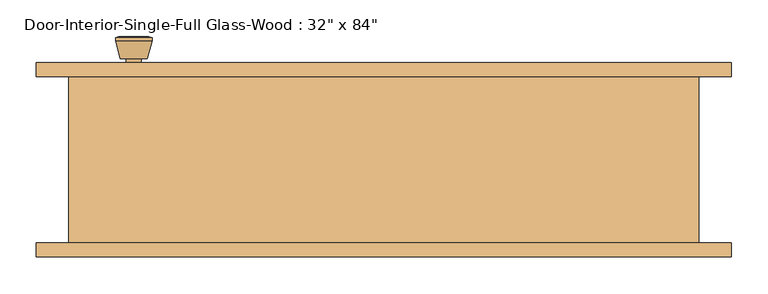
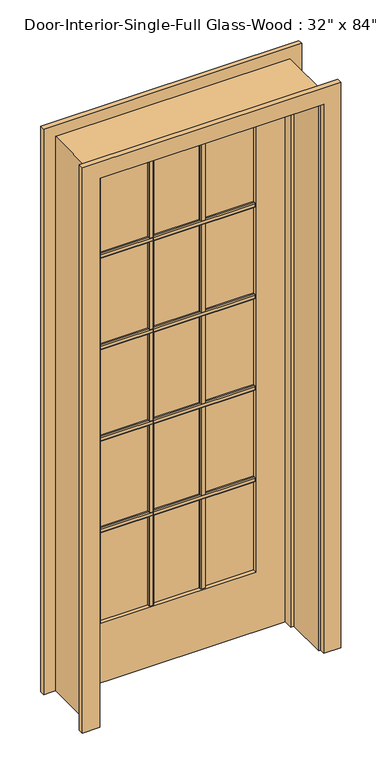
"""IFC4 building model written with IfcOpenShell, lengths in millimetres: door geometry."""

from ifc_helpers import new_model, si_unit, point, frame, frame_2d, origin, place, context, project, spatial, polyline, circle_curve, trimmed, segment, composite_curve, outline, extrude, faceted_brep, source, transform, mapped, element, save
from ifc_brep_helpers import plane_surface, cylinder_surface, revolved_surface, advanced_brep


def door_c0815308(model_context):
    return source(origin(), model_context, "Body", "SolidModel", [
        extrude(outline(polyline([(97.155, 1667.51), (103.505, 1667.51), (106.68, 1664.335), (106.68, 1651.635), (103.505, 1648.46), (97.155, 1648.46), (97.155, 1667.51)])), frame((-285.75, 0.0, 0.0), z_axis=(1.0, 0.0, 0.0), x_axis=(0.0, 1.0, 0.0)), (0.0, 0.0, 1.0), 571.5),
        extrude(outline(polyline([(97.155, 1310.9575), (103.505, 1310.9575), (106.68, 1307.7825), (106.68, 1295.0825), (103.505, 1291.9075), (97.155, 1291.9075), (97.155, 1310.9575)])), frame((-285.75, 0.0, 0.0), z_axis=(1.0, 0.0, 0.0), x_axis=(0.0, 1.0, 0.0)), (0.0, 0.0, 1.0), 571.5),
        extrude(outline(polyline([(97.155, 954.405), (103.505, 954.405), (106.68, 951.23), (106.68, 938.53), (103.505, 935.355), (97.155, 935.355), (97.155, 954.405)])), frame((-285.75, 0.0, 0.0), z_axis=(1.0, 0.0, 0.0), x_axis=(0.0, 1.0, 0.0)), (0.0, 0.0, 1.0), 571.5),
        extrude(outline(polyline([(97.155, 597.8525), (103.505, 597.8525), (106.68, 594.6775), (106.68, 581.9775), (103.505, 578.8025), (97.155, 578.8025), (97.155, 597.8525)])), frame((-285.75, 0.0, 0.0), z_axis=(1.0, 0.0, 0.0), x_axis=(0.0, 1.0, 0.0)), (0.0, 0.0, 1.0), 571.5),
        extrude(outline(polyline([(85.725, 97.155), (85.725, 103.505), (88.9, 106.68), (101.6, 106.68), (104.775, 103.505), (104.775, 97.155), (85.725, 97.155)])), frame((0.0, 0.0, 231.775), z_axis=(0.0, 0.0, 1.0), x_axis=(1.0, 0.0, 0.0)), (0.0, 0.0, 1.0), 1782.7625),
        extrude(outline(polyline([(-104.775, 97.155), (-104.775, 103.505), (-101.6, 106.68), (-88.9, 106.68), (-85.725, 103.505), (-85.725, 97.155), (-104.775, 97.155)])), frame((0.0, 0.0, 231.775), z_axis=(0.0, 0.0, 1.0), x_axis=(1.0, 0.0, 0.0)), (0.0, 0.0, 1.0), 1782.7625),
        extrude(outline(polyline([(90.17, 1667.51), (90.17, 1648.46), (83.82, 1648.46), (80.645, 1651.635), (80.645, 1664.335), (83.82, 1667.51), (90.17, 1667.51)])), frame((-285.75, 0.0, 0.0), z_axis=(1.0, 0.0, 0.0), x_axis=(0.0, 1.0, 0.0)), (0.0, 0.0, 1.0), 571.5),
        extrude(outline(polyline([(90.17, 1310.9575), (90.17, 1291.9075), (83.82, 1291.9075), (80.645, 1295.0825), (80.645, 1307.7825), (83.82, 1310.9575), (90.17, 1310.9575)])), frame((-285.75, 0.0, 0.0), z_axis=(1.0, 0.0, 0.0), x_axis=(0.0, 1.0, 0.0)), (0.0, 0.0, 1.0), 571.5),
        extrude(outline(polyline([(90.17, 954.405), (90.17, 935.355), (83.82, 935.355), (80.645, 938.53), (80.645, 951.23), (83.82, 954.405), (90.17, 954.405)])), frame((-285.75, 0.0, 0.0), z_axis=(1.0, 0.0, 0.0), x_axis=(0.0, 1.0, 0.0)), (0.0, 0.0, 1.0), 571.5),
        extrude(outline(polyline([(90.17, 597.8525), (90.17, 578.8025), (83.82, 578.8025), (80.645, 581.9775), (80.645, 594.6775), (83.82, 597.8525), (90.17, 597.8525)])), frame((-285.75, 0.0, 0.0), z_axis=(1.0, 0.0, 0.0), x_axis=(0.0, 1.0, 0.0)), (0.0, 0.0, 1.0), 571.5),
        extrude(outline(polyline([(85.725, 90.17), (104.775, 90.17), (104.775, 83.82), (101.6, 80.645), (88.9, 80.645), (85.725, 83.82), (85.725, 90.17)])), frame((0.0, 0.0, 231.775), z_axis=(0.0, 0.0, 1.0), x_axis=(1.0, 0.0, 0.0)), (0.0, 0.0, 1.0), 1782.7625),
        extrude(outline(polyline([(-104.775, 90.17), (-85.725, 90.17), (-85.725, 83.82), (-88.9, 80.645), (-101.6, 80.645), (-104.775, 83.82), (-104.775, 90.17)])), frame((0.0, 0.0, 231.775), z_axis=(0.0, 0.0, 1.0), x_axis=(1.0, 0.0, 0.0)), (0.0, 0.0, 1.0), 1782.7625),
        advanced_brep(
        [(-342.9, 70.2, 914.4), (-332.9, 70.2, 914.4), (-352.9, 70.2, 914.4), (-322.4241324, 21.2, 914.4), (-342.9, 21.2, 914.4), (-363.3758676, 21.2, 914.4), (-317.9, 23.0278681, 914.4), (-367.9, 23.0278681, 914.4), (-317.9, 26.4915463, 914.4), (-367.9, 26.4915463, 914.4), (-324.263764, 51.2, 914.4), (-361.536236, 51.2, 914.4), (-332.9, 51.2, 914.4), (-352.9, 51.2, 914.4)],
        [
            (0, 1),
            (1, 2, circle_curve(frame((-342.9, 70.2, 914.4), z_axis=(0.0, 1.0, 0.0), x_axis=(-1.0, 0.0, 0.0)), 10.0)),
            (2, 0),
            (2, 1, circle_curve(frame((-342.9, 70.2, 914.4), z_axis=(0.0, 1.0, 0.0), x_axis=(-1.0, 0.0, 0.0)), 10.0)),
            (3, 4),
            (4, 5),
            (5, 3, circle_curve(frame((-342.9, 21.2, 914.4), z_axis=(0.0, -1.0, 0.0), x_axis=(-1.0, 0.0, 0.0)), 20.4758676)),
            (3, 5, circle_curve(frame((-342.9, 21.2, 914.4), z_axis=(0.0, -1.0, 0.0), x_axis=(-1.0, 0.0, 0.0)), 20.4758676)),
            (6, 3),
            (5, 7),
            (7, 6, circle_curve(frame((-342.9, 23.0278681, 914.4), z_axis=(0.0, -1.0, 0.0), x_axis=(-1.0, 0.0, 0.0)), 25.0)),
            (6, 7, circle_curve(frame((-342.9, 23.0278681, 914.4), z_axis=(0.0, -1.0, 0.0), x_axis=(-1.0, 0.0, 0.0)), 25.0)),
            (8, 6),
            (7, 9),
            (9, 8, circle_curve(frame((-342.9, 26.4915463, 914.4), z_axis=(0.0, -1.0, 0.0), x_axis=(-1.0, 0.0, 0.0)), 25.0)),
            (8, 9, circle_curve(frame((-342.9, 26.4915463, 914.4), z_axis=(0.0, -1.0, 0.0), x_axis=(-1.0, 0.0, 0.0)), 25.0)),
            (10, 8),
            (9, 11),
            (11, 10, circle_curve(frame((-342.9, 51.2, 914.4), z_axis=(0.0, -1.0, 0.0), x_axis=(-1.0, 0.0, 0.0)), 18.636236)),
            (10, 11, circle_curve(frame((-342.9, 51.2, 914.4), z_axis=(0.0, -1.0, 0.0), x_axis=(-1.0, 0.0, 0.0)), 18.636236)),
            (12, 10),
            (11, 13),
            (13, 12, circle_curve(frame((-342.9, 51.2, 914.4), z_axis=(0.0, -1.0, 0.0), x_axis=(-1.0, 0.0, 0.0)), 10.0)),
            (12, 13, circle_curve(frame((-342.9, 51.2, 914.4), z_axis=(0.0, -1.0, 0.0), x_axis=(-1.0, 0.0, 0.0)), 10.0)),
            (1, 12),
            (13, 2),
        ],
        [
            plane_surface(frame((-342.9, 70.2, 914.4), z_axis=(0.0, 1.0, 0.0), x_axis=(-1.0, 0.0, 0.0))),
            plane_surface(frame((-342.9, 21.2, 914.4), z_axis=(0.0, -1.0, 0.0), x_axis=(-1.0, 0.0, 0.0))),
            revolved_surface(polyline([(-363.3758676, 21.2, 914.4), (-367.9, 23.0278681, 914.4)]), (-342.9, 70.2, 914.4), (0.0, 1.0, 0.0)),
            cylinder_surface(frame((-342.9, 70.2, 914.4), z_axis=(0.0, 1.0, 0.0), x_axis=(-1.0, 0.0, 0.0)), 25.0),
            revolved_surface(polyline([(-367.9, 26.4915463, 914.4), (-361.536236, 51.2, 914.4)]), (-342.9, 70.2, 914.4), (0.0, 1.0, 0.0)),
            plane_surface(frame((-342.9, 51.2, 914.4), z_axis=(0.0, 1.0, 0.0), x_axis=(-1.0, 0.0, 0.0))),
            cylinder_surface(frame((-342.9, 70.2, 914.4), z_axis=(0.0, 1.0, 0.0), x_axis=(-1.0, 0.0, 0.0)), 10.0),
        ],
        [
            (0, [[1, 2, 3]]),
            (0, [[-3, 4, -1]]),
            (1, [[5, 6, 7]]),
            (1, [[-6, -5, 8]]),
            (2, [[9, -7, 10, 11]]),
            (2, [[-10, -8, -9, 12]]),
            (3, [[13, -11, 14, 15]]),
            (3, [[-14, -12, -13, 16]]),
            (4, [[17, -15, 18, 19]]),
            (4, [[-18, -16, -17, 20]]),
            (5, [[21, -19, 22, 23]]),
            (5, [[-22, -20, -21, 24]]),
            (6, [[25, -23, 26, -2]]),
            (6, [[-26, -24, -25, -4]]),
        ],
    ),
        extrude(outline(composite_curve([segment(trimmed(circle_curve(frame_2d((914.4, -342.9)), 30.0), [point((914.4, -372.9))], [point((914.4, -312.9))], False, "CARTESIAN"), True, "CONTINUOUS"), segment(trimmed(circle_curve(frame_2d((914.4, -342.9)), 30.0), [point((914.4, -312.9))], [point((914.4, -372.9))], False, "CARTESIAN"), True, "CONTINUOUS")], self_intersect=False)), frame((0.0, 70.2, 0.0), z_axis=(0.0, 1.0, 0.0), x_axis=(0.0, 0.0, 1.0)), (0.0, 0.0, 1.0), 6.0),
        advanced_brep(
        [(-342.9, 117.125, 914.4), (-352.9, 117.125, 914.4), (-332.9, 117.125, 914.4), (-322.4241324, 166.125, 914.4), (-363.3758676, 166.125, 914.4), (-342.9, 166.125, 914.4), (-317.9, 164.2971319, 914.4), (-367.9, 164.2971319, 914.4), (-317.9, 160.8334537, 914.4), (-367.9, 160.8334537, 914.4), (-324.263764, 136.125, 914.4), (-361.536236, 136.125, 914.4), (-332.9, 136.125, 914.4), (-352.9, 136.125, 914.4)],
        [
            (0, 1),
            (1, 2, circle_curve(frame((-342.9, 117.125, 914.4), z_axis=(0.0, -1.0, 0.0), x_axis=(-1.0, 0.0, 0.0)), 10.0)),
            (2, 0),
            (2, 1, circle_curve(frame((-342.9, 117.125, 914.4), z_axis=(0.0, -1.0, 0.0), x_axis=(-1.0, 0.0, 0.0)), 10.0)),
            (3, 4, circle_curve(frame((-342.9, 166.125, 914.4), z_axis=(0.0, 1.0, 0.0), x_axis=(-1.0, 0.0, 0.0)), 20.4758676)),
            (4, 5),
            (5, 3),
            (4, 3, circle_curve(frame((-342.9, 166.125, 914.4), z_axis=(0.0, 1.0, 0.0), x_axis=(-1.0, 0.0, 0.0)), 20.4758676)),
            (6, 7, circle_curve(frame((-342.9, 164.2971319, 914.4), z_axis=(0.0, 1.0, 0.0), x_axis=(-1.0, 0.0, 0.0)), 25.0)),
            (7, 4),
            (3, 6),
            (7, 6, circle_curve(frame((-342.9, 164.2971319, 914.4), z_axis=(0.0, 1.0, 0.0), x_axis=(-1.0, 0.0, 0.0)), 25.0)),
            (8, 9, circle_curve(frame((-342.9, 160.8334537, 914.4), z_axis=(0.0, 1.0, 0.0), x_axis=(-1.0, 0.0, 0.0)), 25.0)),
            (9, 7),
            (6, 8),
            (9, 8, circle_curve(frame((-342.9, 160.8334537, 914.4), z_axis=(0.0, 1.0, 0.0), x_axis=(-1.0, 0.0, 0.0)), 25.0)),
            (10, 11, circle_curve(frame((-342.9, 136.125, 914.4), z_axis=(0.0, 1.0, 0.0), x_axis=(-1.0, 0.0, 0.0)), 18.636236)),
            (11, 9),
            (8, 10),
            (11, 10, circle_curve(frame((-342.9, 136.125, 914.4), z_axis=(0.0, 1.0, 0.0), x_axis=(-1.0, 0.0, 0.0)), 18.636236)),
            (12, 13, circle_curve(frame((-342.9, 136.125, 914.4), z_axis=(0.0, 1.0, 0.0), x_axis=(-1.0, 0.0, 0.0)), 10.0)),
            (13, 11),
            (10, 12),
            (13, 12, circle_curve(frame((-342.9, 136.125, 914.4), z_axis=(0.0, 1.0, 0.0), x_axis=(-1.0, 0.0, 0.0)), 10.0)),
            (1, 13),
            (12, 2),
        ],
        [
            plane_surface(frame((-342.9, 117.125, 914.4), z_axis=(0.0, -1.0, 0.0), x_axis=(-1.0, 0.0, 0.0))),
            plane_surface(frame((-342.9, 166.125, 914.4), z_axis=(0.0, 1.0, 0.0), x_axis=(-1.0, 0.0, 0.0))),
            revolved_surface(polyline([(-363.3758676, 166.125, 914.4), (-367.9, 164.2971319, 914.4)]), (-342.9, 117.125, 914.4), (0.0, -1.0, 0.0)),
            cylinder_surface(frame((-342.9, 117.125, 914.4), z_axis=(0.0, -1.0, 0.0), x_axis=(-1.0, 0.0, 0.0)), 25.0),
            revolved_surface(polyline([(-367.9, 160.8334537, 914.4), (-361.536236, 136.125, 914.4)]), (-342.9, 117.125, 914.4), (0.0, -1.0, 0.0)),
            plane_surface(frame((-342.9, 136.125, 914.4), z_axis=(0.0, -1.0, 0.0), x_axis=(-1.0, 0.0, 0.0))),
            cylinder_surface(frame((-342.9, 117.125, 914.4), z_axis=(0.0, -1.0, 0.0), x_axis=(-1.0, 0.0, 0.0)), 10.0),
        ],
        [
            (0, [[1, 2, 3]]),
            (0, [[-3, 4, -1]]),
            (1, [[5, 6, 7]]),
            (1, [[8, -7, -6]]),
            (2, [[9, 10, -5, 11]]),
            (2, [[12, -11, -8, -10]]),
            (3, [[13, 14, -9, 15]]),
            (3, [[16, -15, -12, -14]]),
            (4, [[17, 18, -13, 19]]),
            (4, [[20, -19, -16, -18]]),
            (5, [[21, 22, -17, 23]]),
            (5, [[24, -23, -20, -22]]),
            (6, [[-2, 25, -21, 26]]),
            (6, [[-4, -26, -24, -25]]),
        ],
    ),
        extrude(outline(composite_curve([segment(trimmed(circle_curve(frame_2d((914.4, -342.9)), 30.0), [point((914.4, -372.9))], [point((914.4, -312.9))], False, "CARTESIAN"), True, "CONTINUOUS"), segment(trimmed(circle_curve(frame_2d((914.4, -342.9)), 30.0), [point((914.4, -312.9))], [point((914.4, -372.9))], False, "CARTESIAN"), True, "CONTINUOUS")], self_intersect=False)), frame((0.0, 111.125, 0.0), z_axis=(0.0, 1.0, 0.0), x_axis=(0.0, 0.0, 1.0)), (0.0, 0.0, 1.0), 6.0),
        faceted_brep([(431.8, 111.125, 0.0), (431.8, -117.475, 0.0), (406.4, -117.475, 0.0), (406.4, 41.275, 0.0), (393.7, 41.275, 0.0), (393.7, 76.2, 0.0), (406.4, 76.2, 0.0), (406.4, 111.125, 0.0), (431.8, 111.125, 2159.0), (431.8, -117.475, 2159.0), (-431.8, -117.475, 2159.0), (-431.8, -117.475, 0.0), (-406.4, -117.475, 0.0), (-406.4, -117.475, 2133.6), (406.4, -117.475, 2133.6), (406.4, 41.275, 2133.6), (-406.4, 41.275, 2133.6), (-406.4, 41.275, 0.0), (-393.7, 41.275, 0.0), (-393.7, 41.275, 2120.9), (393.7, 41.275, 2120.9), (393.7, 76.2, 2120.9), (-393.7, 76.2, 2120.9), (-393.7, 76.2, 0.0), (-406.4, 76.2, 0.0), (-406.4, 76.2, 2133.6), (406.4, 76.2, 2133.6), (406.4, 111.125, 2133.6), (-406.4, 111.125, 2133.6), (-406.4, 111.125, 0.0), (-431.8, 111.125, 0.0), (-431.8, 111.125, 2159.0)], [[[0, 1, 2, 3, 4, 5, 6, 7]], [[1, 0, 8, 9]], [[2, 1, 9, 10, 11, 12, 13, 14]], [[3, 2, 14, 15]], [[4, 3, 15, 16, 17, 18, 19, 20]], [[5, 4, 20, 21]], [[6, 5, 21, 22, 23, 24, 25, 26]], [[7, 6, 26, 27]], [[0, 7, 27, 28, 29, 30, 31, 8]], [[9, 8, 31, 10]], [[15, 14, 13, 16]], [[21, 20, 19, 22]], [[27, 26, 25, 28]], [[30, 29, 24, 23, 18, 17, 12, 11]], [[10, 31, 30, 11]], [[16, 13, 12, 17]], [[22, 19, 18, 23]], [[28, 25, 24, 29]]]),
        extrude(outline(polyline([(2133.6, -406.4), (0.0, -406.4), (0.0, 406.4), (2133.6, 406.4), (2133.6, -406.4)]), holes=[polyline([(2014.5375, -285.75), (2014.5375, 285.75), (231.775, 285.75), (231.775, -285.75), (2014.5375, -285.75)])]), frame((0.0, 76.2, 0.0), z_axis=(0.0, 1.0, 0.0), x_axis=(0.0, 0.0, 1.0)), (0.0, 0.0, 1.0), 34.925),
        extrude(outline(polyline([(285.75, 90.17), (-285.75, 90.17), (-285.75, 97.155), (285.75, 97.155), (285.75, 90.17)])), frame((0.0, 0.0, 231.775), z_axis=(0.0, 0.0, 1.0), x_axis=(1.0, 0.0, 0.0)), (0.0, 0.0, 1.0), 1782.7625),
        extrude(outline(polyline([(0.0, 412.75), (0.0, 476.25), (2203.45, 476.25), (2203.45, -476.25), (0.0, -476.25), (0.0, -412.75), (2139.95, -412.75), (2139.95, 412.75), (0.0, 412.75)])), frame((0.0, 111.125, 0.0), z_axis=(0.0, 1.0, 0.0), x_axis=(0.0, 0.0, 1.0)), (0.0, 0.0, 1.0), 19.05),
        extrude(outline(polyline([(0.0, 412.75), (0.0, 476.25), (2203.45, 476.25), (2203.45, -476.25), (0.0, -476.25), (0.0, -412.75), (2139.95, -412.75), (2139.95, 412.75), (0.0, 412.75)])), frame((0.0, -136.525, 0.0), z_axis=(0.0, 1.0, 0.0), x_axis=(0.0, 0.0, 1.0)), (0.0, 0.0, 1.0), 19.05),
    ])


if __name__ == "__main__":
    model = new_model("IFC4")
    model_context = context("Model", 3, world=origin())
    ifc_project = project(units=[si_unit("LENGTHUNIT", "METRE", prefix="MILLI")], contexts=[model_context])
    site = spatial("IfcSite", under=ifc_project)
    building = spatial("IfcBuilding", under=site)
    placement = place(None, origin())
    door_shape = door_c0815308(model_context)
    element("IfcDoor", 1, ObjectType="Door-Interior-Single-Full Glass-Wood : 32\" x 84\"", at=placement, inside=building, context=model_context, shape_type="MappedRepresentation", body=[
        mapped(door_shape, transform((0.0, 0.0, 0.0), x_axis=(1.0, 0.0, 0.0), y_axis=(0.0, 1.0, 0.0), z_axis=(0.0, 0.0, 1.0))),
    ])
    save(model, "model.ifc")

# Revit data of these elements
# Type "Door-Interior-Single-Full Glass-Wood : 32\" x 84\""
#   Type Mark = "9"
#   Assembly Code = "C1020300"
#   Analytic Construction = "Wood frame with single clear glass"
#   Top Rail = 0' - 4 11/16"
#   Thickness = 0' - 1 3/8"
#   Thermal Resistance (R) = 1.0102 (h·ft²·°F)/BTU
#   Swing Angle [instance default] = 90.00°
#   Stiles = 0' - 4 3/4"
#   Rough Width = 2' - 10"
#   Rough Height = 7' - 1"
#   Height = 7' - 0"
#   Width = 2' - 8"
#   Heat Transfer Coefficient (U) = 0.9900 BTU/(h·ft²·°F)
#   Bottom Rail = 0' - 9 1/8"
#   Show Grill [instance default] = yes
#   Trim Material = Cherry
#   Panel Material = Cherry
#   Frame Material = Cherry
#   Door Handle Material = Aluminum
#   Visual Light Transmittance = 0
#   Solar Heat Gain Coefficient = 0
#   Wall Closure = (empty or 0)
#   Function = (empty or 0)
# Element 1 (IfcDoor, "Door-Interior-Single-Full Glass-Wood : 32\" x 84\"")
#   Materials on its faces: "Cherry", "Aluminum", "Glass"
# Materials
#   "Cherry": class "Wood", colour RGB 226 177 128, transparency 0, Description = "Prunus Serotina", Cost = 0
#   "Aluminum": class "Metal", colour RGB 247 247 247, transparency 0, Description = "Aluminum 6061", Cost = 0
#   "Glass": class "Glass", colour RGB 0 128 192, transparency 0.75, Description = "Soda Lime Glass", Cost = 0
